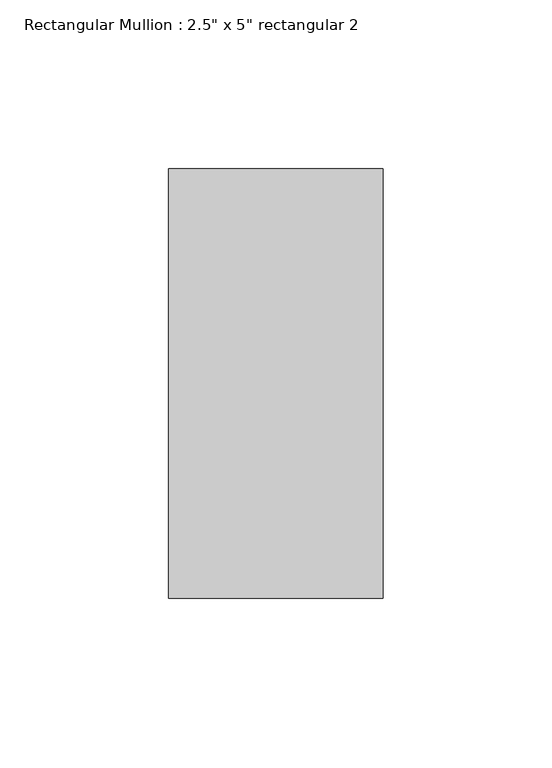
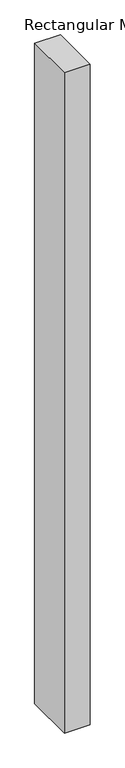
"""IFC4 building model written with IfcOpenShell, lengths in millimetres: member geometry."""

from ifc_helpers import new_model, si_unit, frame, origin, place, context, project, spatial, polyline, outline, extrude, source, transform, mapped, element, save


def member_58564e40(model_context):
    return source(origin(), model_context, "Body", "SweptSolid", [
        extrude(outline(polyline([(31.75, 63.5), (31.75, -63.5), (-31.75, -63.5), (-31.75, 63.5), (31.75, 63.5)])), frame((0.0, 0.0, -1720.9224616), z_axis=(0.0, 0.0, 1.0), x_axis=(1.0, 0.0, 0.0)), (0.0, 0.0, 1.0), 1720.9224616),
    ])


if __name__ == "__main__":
    model = new_model("IFC4")
    model_context = context("Model", 3, world=origin())
    ifc_project = project(units=[si_unit("LENGTHUNIT", "METRE", prefix="MILLI")], contexts=[model_context])
    site = spatial("IfcSite", under=ifc_project)
    building = spatial("IfcBuilding", under=site)
    placement = place(None, origin())
    member_shape = member_58564e40(model_context)
    element("IfcMember", 1, ObjectType="Rectangular Mullion : 2.5\" x 5\" rectangular 2", at=placement, inside=building, context=model_context, shape_type="MappedRepresentation", body=[
        mapped(member_shape, transform((0.0, 0.0, 0.0), x_axis=(1.0, 0.0, 0.0), y_axis=(0.0, 1.0, 0.0), z_axis=(0.0, 0.0, 1.0))),
    ])
    save(model, "model.ifc")

# Revit data of these elements
# Type "Rectangular Mullion : 2.5\" x 5\" rectangular 2"
#   built-in parameter 1007304 = 0.416667 (stored number, unit not read)
#   built-in parameter 1007301 = 0.104167 (stored number, unit not read)
#   built-in parameter 1007300 = 0.104167 (stored number, unit not read)
